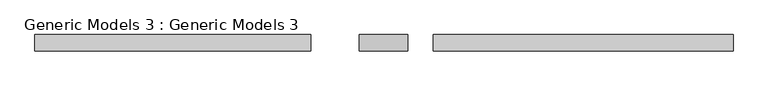
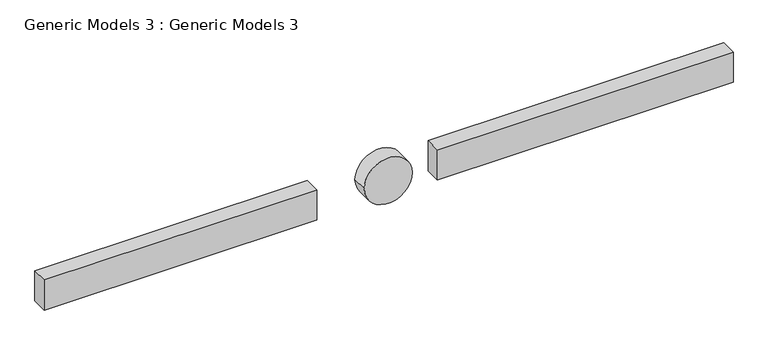
"""IFC4 building model written with IfcOpenShell, lengths in millimetres: proxy geometry, Generic Models 3 : Generic Models 3."""

from ifc_helpers import new_model, si_unit, point, frame, frame_2d, origin, place, context, project, spatial, polyline, circle_curve, trimmed, segment, composite_curve, outline, extrude, source, transform, mapped, element, save


def generic_models_3_generic_models_3_f3c11b88(model_context):
    return source(origin(), model_context, "Body", "SweptSolid", [
        extrude(outline(polyline([(-2343.138363, -2327.5868249), (-7524.738363, -2327.5868249), (-7524.738363, -2022.7868249), (-2343.138363, -2022.7868249), (-2343.138363, -2327.5868249)])), frame((0.0, 0.0, 9965.8546615), z_axis=(0.0, 0.0, 1.0), x_axis=(1.0, 0.0, 0.0)), (0.0, 0.0, 1.0), 609.6),
        extrude(outline(polyline([(5582.448676, -2327.5868249), (-43.2953031, -2327.5868249), (-43.2953031, -2022.7868249), (5582.448676, -2022.7868249), (5582.448676, -2327.5868249)])), frame((0.0, 0.0, 9965.8546615), z_axis=(0.0, 0.0, 1.0), x_axis=(1.0, 0.0, 0.0)), (0.0, 0.0, 1.0), 609.6),
        extrude(outline(composite_curve([segment(trimmed(circle_curve(frame_2d((10283.2670375, -977.9599678)), 457.2), [point((10283.2670375, -1435.1599678))], [point((10283.2670375, -520.7599678))], False, "CARTESIAN"), True, "CONTINUOUS"), segment(trimmed(circle_curve(frame_2d((10283.2670375, -977.9599678)), 457.2), [point((10283.2670375, -520.7599678))], [point((10283.2670375, -1435.1599678))], False, "CARTESIAN"), True, "CONTINUOUS")], self_intersect=False)), frame((0.0, -2327.5868249, 0.0), z_axis=(0.0, 1.0, 0.0), x_axis=(0.0, 0.0, 1.0)), (0.0, 0.0, 1.0), 304.8),
    ])


if __name__ == "__main__":
    model = new_model("IFC4")
    model_context = context("Model", 3, world=origin())
    ifc_project = project(units=[si_unit("LENGTHUNIT", "METRE", prefix="MILLI")], contexts=[model_context])
    site = spatial("IfcSite", under=ifc_project)
    building = spatial("IfcBuilding", under=site)
    placement = place(None, origin())
    generic_models_3_generic_models_3_shape = generic_models_3_generic_models_3_f3c11b88(model_context)
    element("IfcBuildingElementProxy", 1, Name="Generic Models 3 : Generic Models 3", ObjectType="Generic Models 3 : Generic Models 3", at=placement, inside=building, context=model_context, shape_type="MappedRepresentation", body=[
        mapped(generic_models_3_generic_models_3_shape, transform((0.0, 0.0, 0.0), x_axis=(1.0, 0.0, 0.0), y_axis=(0.0, 1.0, 0.0), z_axis=(0.0, 0.0, 1.0))),
    ])
    save(model, "model.ifc")

# Revit data of these elements
# Element 1 (IfcBuildingElementProxy, "Generic Models 3 : Generic Models 3")
#   Materials on its faces: "sheets", "Parking Stripe"
# Materials
#   "sheets": colour RGB 200 195 176, transparency 0, Cost = 0
#   "Parking Stripe": class "Paint", colour RGB 250 250 91, transparency 0, Cost = 0
